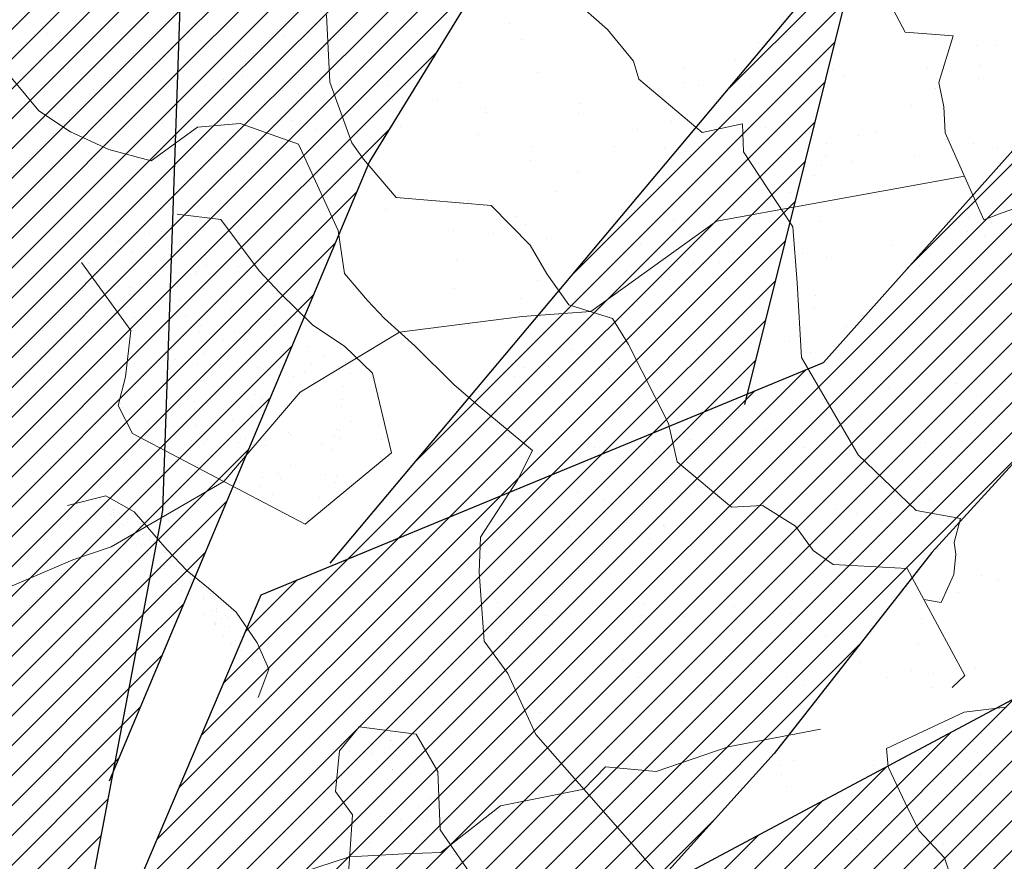
# Model space of a CAD drawing. Units: inches. Extents: x 1986 to 21484, y -1816 to 2016.
# Tile 73 of 85: x 3669.485 to 3676.656, y 1888.787 to 1894.917. Entities that reach past the tile are written whole.
import ezdxf

# ---------------------------------------------------------------- set-up
doc = ezdxf.new("R2010")
doc.units = ezdxf.units.IN
doc.layers.add('L-PLNT', color=84, linetype='Continuous', lineweight=13)
doc.layers.add('vfolhas', color=114, linetype='Continuous', lineweight=5)
doc.layers.add('vfolha2', color=110, linetype='Continuous')
doc.layers.add('vfolhas2', color=102, linetype='Continuous')
pattern_1 = [(45, (-2446.5133113, 50.986076), (-0.004419417382, 0.004419417382), [])]

# ---------------------------------------------------------------- blocks, each defined once
blk = doc.blocks.new('arbusto_PB_verde_grande')
at = {"layer": 'vfolha2'}
h = blk.add_hatch(dxfattribs=at)
h.set_pattern_fill('ANSI31', color=256, scale=0.05, style=0)
h.set_pattern_definition(pattern_1)
h.paths.add_polyline_path([(0.02944, 0.35651), (0.00028, 0.09048), (0.02625, -0.03934), (0.047, 0.06233), (0.06189, 0.09731), (0.09372, 0.26573), (0.09955, 0.43473), (0.08789, 0.61313), (0.0645, 0.72266), (0.04988, 0.6851), (0.0236, 0.51294)])
h.paths.add_polyline_path([(0.30106, 0.43789), (0.14225, 0.24871), (0.26685, 0.30022)])
h.paths.add_polyline_path([(0.37995, 0.22817), (0.23697, 0.15193), (0.18428, 0.09364), (0.11122, 0.04358), (0.02625, -0.03934), (0.28061, 0.04667), (0.36829, 0.07798), (0.46756, 0.11239), (0.61068, 0.19376), (0.71585, 0.27823), (0.55813, 0.25948)])
h.paths.add_polyline_path([(0.56101, -0.29441), (0.72752, -0.32573), (0.59024, -0.2412), (0.42962, -0.15982), (0.02625, -0.03934), (0.14922, -0.14107), (0.18838, -0.16604), (0.41501, -0.24435)])
h.paths.add_polyline_path([(-0.27429, -0.44776), (-0.30352, -0.72628), (-0.23923, -0.64175), (-0.15457, -0.45716), (0.02625, -0.03934), (-0.16328, -0.25376)])
h.paths.add_polyline_path([(-0.51963, -0.24744), (-0.67736, -0.32573), (-0.59558, -0.35072), (-0.40574, -0.32882), (-0.21007, -0.20995), (0.02625, -0.03934), (-0.14874, -0.06595), (-0.31518, -0.09101), (-0.41452, -0.15048)])
h.paths.add_polyline_path([(-0.52546, 0.25007), (-0.70947, 0.24698), (-0.51963, 0.1093), (-0.32979, 0.02167), (-0.07567, -0.0128), (-0.04234, -0.02148), (-0.35024, 0.1312)])
at = {"layer": 'vfolhas'}
h = blk.add_hatch(dxfattribs=at)
h.set_pattern_fill('ANSI31', color=256, scale=0.05, style=0)
h.set_pattern_definition(pattern_1)
h.paths.add_polyline_path([(-0.07279, 0.50669), (-0.18085, 0.65063), (-0.2334, 0.67253), (-0.20712, 0.53176), (-0.10785, 0.25007), (0.02625, -0.03934), (0.00028, 0.09048), (0.00816, 0.16241), (-0.04939, 0.29079)])
h.paths.add_polyline_path([(0.09902, 0.41929), (0.09372, 0.26573), (0.07906, 0.18814), (0.15506, 0.36901), (0.26606, 0.5505), (0.28356, 0.63504), (0.2485, 0.68819), (0.25145, 0.63504), (0.20178, 0.54426)])
h.paths.add_polyline_path([(0.12295, 0.24073), (0.047, 0.06233), (0.02625, -0.03934), (0.11122, 0.04358), (0.18428, 0.09364), (0.27478, 0.19376), (0.3215, 0.25323), (0.44129, 0.38467), (0.47634, 0.57866), (0.41789, 0.45347), (0.28939, 0.30954)])
h.paths.add_polyline_path([(0.58145, -0.03779), (0.70707, 0.01536), (0.78591, 0.04667), (0.74796, 0.06549), (0.62818, 0.08423), (0.52595, 0.09048), (0.39745, 0.04358), (0.02625, -0.03934), (0.25728, -0.03154), (0.43834, -0.0347)])
h.paths.add_polyline_path([(0.52022, -0.03647), (0.43834, -0.0347), (0.25728, -0.03154), (0.02625, -0.03934), (0.17964, -0.08515), (0.53768, -0.13167), (0.69541, -0.15357), (0.78591, -0.07852), (0.70413, -0.10042)])
h.paths.add_polyline_path([(0.27189, -0.21929), (0.14922, -0.14107), (0.02625, -0.03934), (0.15794, -0.31007), (0.29522, -0.42585), (0.41789, -0.49157), (0.56396, -0.56669), (0.5114, -0.48532), (0.39456, -0.34139)])
h.paths.add_polyline_path([(-0.05818, -0.47591), (-0.02312, -0.61984), (0.047, -0.80134), (0.08494, -0.59794), (0.07911, -0.4071), (0.03527, -0.25376), (0.02625, -0.03934), (-0.03773, -0.26001)])
h.paths.add_polyline_path([(-0.24218, 0.14054), (-0.11073, 0.06858), (0.02625, -0.03934), (-0.04235, 0.10871), (-0.21007, 0.23757), (-0.36485, 0.33145), (-0.47874, 0.40341), (-0.54303, 0.46288), (-0.49041, 0.33145), (-0.39408, 0.22192)])
at = {"layer": 'vfolha2'}
for p, q in [((0.14339, 0.25007), (0.30106, 0.43789)), ((0.30106, 0.43789), (0.26606, 0.29704)), ((0.09955, 0.43473), (0.09372, 0.26573)), ((0.23697, 0.15193), (0.37995, 0.22817))]:
    blk.add_line(p, q, dxfattribs=at)
at = {"layer": 'vfolhas2'}
for p, q in [((0.26606, 0.5505), (0.15506, 0.36901)), ((0.28939, 0.30954), (0.41789, 0.45347)), ((0.44129, 0.38467), (0.3215, 0.25323)), ((0.15506, 0.36901), (0.07795, 0.18551)), ((0.12295, 0.24073), (0.28939, 0.30954)), ((0.09372, 0.26573), (0.06189, 0.09731)), ((0.3215, 0.25323), (0.27478, 0.19376)), ((0.047, 0.06233), (0.12295, 0.24073)), ((0.27478, 0.19376), (0.18428, 0.09364))]:
    blk.add_line(p, q, dxfattribs=at)
blk = doc.blocks.new('PLANT-SHRUB')
for p, q in [((2155.3771, 1891.3729), (2155.4666, 1891.568)), ((2155.3771, 1891.1047), (2155.3771, 1891.3729)), ((2155.3155, 1891.2998), (2155.3155, 1891.2998)), ((2154.9383, 1891.2139), (2154.9383, 1891.2139)), ((2155.4084, 1891.1607), (2155.4084, 1891.1607)), ((2154.7698, 1891.1065), (2154.7698, 1891.1065)), ((2155.3283, 1890.934), (2155.3771, 1891.1047)), ((2155.3348, 1891.0932), (2155.3348, 1891.0932)), ((2154.6758, 1890.9774), (2154.6758, 1890.9774)), ((2155.2225, 1890.6089), (2155.3283, 1890.934)), ((2154.3034, 1890.8771), (2154.5474, 1890.6983)), ((2154.8084, 1890.8995), (2154.8084, 1890.8995)), ((2155.2187, 1890.9059), (2155.2187, 1890.9059)), ((2155.4267, 1890.8785), (2155.4267, 1890.8785)), ((2155.8546, 1890.8861), (2155.8546, 1890.8861)), ((2155.7517, 1890.8357), (2155.7517, 1890.8357)), ((2154.937, 1890.7286), (2154.937, 1890.7286)), ((2154.5474, 1890.6983), (2155.1412, 1890.5032)), ((2155.1412, 1890.5032), (2155.2225, 1890.6089)), ((2155.2223, 1890.5996), (2155.2223, 1890.5996)), ((2154.1988, 1889.8984), (2154.3599, 1890.5058)), ((2154.268, 1890.5248), (2154.268, 1890.5248)), ((2154.3599, 1890.5058), (2154.4874, 1890.5058)), ((2154.3599, 1890.5058), (2154.3599, 1890.5058)), ((2155.2904, 1890.5297), (2155.2904, 1890.5297)), ((2154.5893, 1890.41), (2154.5893, 1890.41)), ((2156.1384, 1890.3779), (2156.1384, 1890.3779)), ((2154.5156, 1890.3425), (2154.5156, 1890.3425)), ((2154.6155, 1890.2131), (2154.6155, 1890.2131)), ((2155.8602, 1890.2108), (2155.8602, 1890.2108)), ((2153.7037, 1890.1683), (2153.7037, 1890.1683)), ((2154.447, 1890.1057), (2154.447, 1890.1057)), ((2154.7832, 1890.1294), (2154.7832, 1890.1294)), ((2155.9718, 1889.7054), (2155.3949, 1890.0722)), ((2155.6916, 1890.1034), (2155.6916, 1890.1034)), ((2155.8294, 1890.1161), (2155.8294, 1890.1161)), ((2153.7744, 1890.0612), (2153.7744, 1890.0612)), ((2153.9153, 1889.9136), (2154.1228, 1889.9996)), ((2153.9824, 1890.0338), (2153.9824, 1890.0338)), ((2154.1228, 1889.9996), (2154.1988, 1889.8984)), ((2155.7907, 1890.0592), (2155.7907, 1890.0592)), ((2156.968, 1889.7436), (2156.9795, 1890.0186)), ((2154.1178, 1889.978), (2154.1178, 1889.978)), ((2154.3073, 1889.9911), (2154.3073, 1889.9911)), ((2155.7171, 1889.9917), (2155.7171, 1889.9917)), ((2153.8039, 1889.8174), (2153.9153, 1889.9136)), ((2154.1988, 1889.8984), (2154.1324, 1889.6508)), ((2154.8502, 1889.9196), (2154.8502, 1889.9196)), ((2155.0582, 1889.8922), (2155.0582, 1889.8922)), ((2155.3832, 1889.8494), (2155.3832, 1889.8494)), ((2153.7533, 1889.7466), (2153.8039, 1889.8174)), ((2155.926, 1889.778), (2155.926, 1889.778)), ((2153.6014, 1889.6505), (2153.7533, 1889.7466)), ((2154.2428, 1889.7547), (2154.2428, 1889.7547)), ((2155.2652, 1889.7596), (2155.2652, 1889.7596)), ((2156.1341, 1889.7506), (2156.1341, 1889.7506)), ((2156.3446, 1889.7207), (2156.3446, 1889.7207)), ((2156.459, 1889.7078), (2156.459, 1889.7078)), ((2156.9323, 1888.68), (2156.968, 1889.7436)), ((2153.7961, 1889.386), (2153.6014, 1889.6505)), ((2153.7701, 1889.6594), (2153.7701, 1889.6594)), ((2154.1324, 1889.6508), (2154.5056, 1889.2597)), ((2156.4787, 1889.4784), (2155.9718, 1889.7054)), ((2153.6549, 1889.6011), (2153.6549, 1889.6011)), ((2153.6964, 1889.5919), (2153.6964, 1889.5919)), ((2154.8995, 1889.5988), (2154.8995, 1889.5988)), ((2155.3193, 1889.6272), (2155.3193, 1889.6272)), ((2156.1441, 1889.5965), (2156.1441, 1889.5965)), ((2156.7234, 1889.1989), (2156.4787, 1889.4784)), ((2153.6786, 1889.3982), (2153.6786, 1889.3982)), ((2153.8268, 1888.8023), (2153.7961, 1889.386)), ((2154.758, 1889.3593), (2154.758, 1889.3593)), ((2154.9715, 1889.3086), (2154.9715, 1889.3086)), ((2155.8042, 1889.346), (2155.8042, 1889.346)), ((2156.5207, 1889.2764), (2156.5207, 1889.2764)), ((2153.0481, 1889.2145), (2153.0481, 1889.2145)), ((2153.2986, 1889.2274), (2153.2986, 1889.2274)), ((2154.2928, 1889.2123), (2154.2928, 1889.2123)), ((2154.5056, 1889.2597), (2154.542, 1889.0869)), ((2154.8979, 1889.2411), (2154.8979, 1889.2411)), ((2155.5374, 1889.21), (2155.5374, 1889.21)), ((2156.9502, 1889.2118), (2156.7234, 1889.1989)), ((2156.782, 1889.2077), (2156.782, 1889.2077)), ((2157.475, 1888.8845), (2156.9502, 1889.2118)), ((2152.863, 1889.1464), (2152.863, 1889.1464)), ((2157.9168, 1888.7107), (2157.9866, 1889.1716)), ((2152.8796, 1889.1072), (2152.8796, 1889.1072)), ((2153.4059, 1889.0749), (2153.4059, 1889.0749)), ((2154.1242, 1889.1049), (2154.1242, 1889.1049)), ((2154.542, 1889.0869), (2154.5147, 1888.8686)), ((2155.3689, 1889.1026), (2155.3689, 1889.1026)), ((2156.6135, 1889.1004), (2156.6135, 1889.1004)), ((2153.1714, 1888.9979), (2153.1714, 1888.9979)), ((2153.6139, 1889.0475), (2153.6139, 1889.0475)), ((2153.9388, 1889.0048), (2153.9388, 1889.0048)), ((2155.24, 1888.9895), (2155.24, 1888.9895)), ((2154.2176, 1888.9846), (2154.2176, 1888.9846)), ((2154.4817, 1888.9333), (2154.4817, 1888.9333)), ((2156.173, 1888.9578), (2156.173, 1888.9578)), ((2156.3195, 1888.9506), (2156.3195, 1888.9506)), ((2157.993, 1888.9486), (2157.993, 1888.9486)), ((2152.9509, 1888.9087), (2152.9509, 1888.9087)), ((2154.5001, 1888.8766), (2154.5001, 1888.8766)), ((2154.5147, 1888.8686), (2154.5875, 1888.5957)), ((2154.6897, 1888.9059), (2154.6897, 1888.9059)), ((2155.0147, 1888.8631), (2155.0147, 1888.8631)), ((2156.0993, 1888.8903), (2156.0993, 1888.8903)), ((2158.0239, 1888.8339), (2157.475, 1888.8845)), ((2157.9562, 1888.9149), (2157.9562, 1888.9149)), ((2152.8772, 1888.8412), (2152.8772, 1888.8412)), ((2153.6423, 1888.0035), (2153.8268, 1888.8023)), ((2155.5575, 1888.7917), (2155.5575, 1888.7917)), ((2158.2267, 1888.6574), (2158.0239, 1888.8339)), ((2155.7656, 1888.7643), (2155.7656, 1888.7643)), ((2156.0905, 1888.7215), (2156.0905, 1888.7215)), ((2157.6372, 1888.3894), (2157.9168, 1888.7107)), ((2158.1345, 1888.742), (2158.1345, 1888.742)), ((2156.6334, 1888.65), (2156.6334, 1888.65)), ((2156.7781, 1888.2176), (2156.9323, 1888.68)), ((2158.0268, 1888.6514), (2158.0268, 1888.6514)), ((2158.5318, 1888.4034), (2158.2267, 1888.6574)), ((2152.631, 1888.6232), (2152.631, 1888.6232)), ((2153.3321, 1888.6002), (2153.3321, 1888.6002)), ((2153.6534, 1888.6281), (2153.6534, 1888.6281)), ((2154.5767, 1888.598), (2154.5767, 1888.598)), ((2154.5875, 1888.5957), (2154.7604, 1888.4502)), ((2154.7329, 1888.5892), (2154.7329, 1888.5892)), ((2155.779, 1888.5759), (2155.779, 1888.5759)), ((2155.8214, 1888.5957), (2155.8214, 1888.5957)), ((2156.8014, 1888.5808), (2156.8014, 1888.5808)), ((2156.8414, 1888.6226), (2156.8414, 1888.6226)), ((2157.9425, 1888.5977), (2157.9425, 1888.5977)), ((2158.7555, 1888.6129), (2158.3082, 1888.1939)), ((2154.0787, 1888.4905), (2154.0787, 1888.4905)), ((2154.1524, 1888.558), (2154.1524, 1888.558)), ((2155.7015, 1888.5258), (2155.7015, 1888.5258)), ((2157.8132, 1888.4947), (2157.8132, 1888.4947)), ((2157.8809, 1888.5419), (2157.8809, 1888.5419)), ((2158.358, 1888.5572), (2158.358, 1888.5572)), ((2158.404, 1888.5352), (2158.404, 1888.5352)), ((2152.4794, 1888.4767), (2152.4794, 1888.4767)), ((2154.7604, 1888.4502), (2154.8241, 1887.9369)), ((2154.7604, 1888.4502), (2154.7604, 1888.4502)), ((2157.9172, 1888.481), (2157.9172, 1888.481)), ((2158.0797, 1888.4596), (2158.0797, 1888.4596)), ((2158.3511, 1888.4239), (2158.3511, 1888.4239)), ((2151.8639, 1888.2323), (2151.4605, 1888.408)), ((2157.5673, 1888.0821), (2157.6372, 1888.3894)), ((2158.1219, 1888.357), (2158.1219, 1888.357)), ((2158.1473, 1888.3641), (2158.1473, 1888.3641)), ((2158.1688, 1888.3442), (2158.1688, 1888.3442)), ((2158.1842, 1888.3979), (2158.1842, 1888.3979)), ((2158.4551, 1888.4102), (2158.4551, 1888.4102)), ((2159.4328, 1887.9763), (2158.5318, 1888.4034)), ((2151.9879, 1888.1806), (2151.8639, 1888.2323)), ((2151.9616, 1888.2303), (2151.9616, 1888.2303)), ((2152.0668, 1888.2667), (2152.0668, 1888.2667)), ((2152.1696, 1888.2029), (2152.1696, 1888.2029)), ((2152.7253, 1888.2137), (2152.7253, 1888.2137)), ((2153.1463, 1888.2278), (2153.1463, 1888.2278)), ((2153.97, 1888.2114), (2153.97, 1888.2114)), ((2154.1924, 1888.2145), (2154.1924, 1888.2145)), ((2155.2146, 1888.2092), (2155.2146, 1888.2092)), ((2155.2148, 1888.2194), (2155.2148, 1888.2194)), ((2155.3538, 1888.2072), (2155.3538, 1888.2072)), ((2156.4592, 1888.2069), (2156.4592, 1888.2069)), ((2156.7418, 1887.9274), (2156.7781, 1888.2176)), ((2156.7781, 1888.2176), (2156.7781, 1888.2176)), ((2151.7601, 1887.5256), (2151.9879, 1888.1806)), ((2152.1317, 1888.1581), (2152.1317, 1888.1581)), ((2152.4945, 1888.1601), (2152.4945, 1888.1601)), ((2155.2802, 1888.1397), (2155.2802, 1888.1397)), ((2156.2943, 1888.1805), (2156.2943, 1888.1805)), ((2157.8654, 1888.151), (2157.8654, 1888.151)), ((2157.8683, 1888.1568), (2157.8683, 1888.1568)), ((2157.9484, 1888.1819), (2157.9484, 1888.1819)), ((2158.3082, 1888.1939), (2158.2802, 1887.9844)), ((2152.0581, 1888.0906), (2152.0581, 1888.0906)), ((2152.5568, 1888.1063), (2152.5568, 1888.1063)), ((2153.0374, 1888.0886), (2153.0374, 1888.0886)), ((2153.2454, 1888.0613), (2153.2454, 1888.0613)), ((2153.6809, 1888.1259), (2153.6809, 1888.1259)), ((2153.8014, 1888.1041), (2153.8014, 1888.1041)), ((2155.0461, 1888.1018), (2155.0461, 1888.1018)), ((2156.2907, 1888.0996), (2156.2907, 1888.0996)), ((2157.8329, 1887.7609), (2157.5673, 1888.0821)), ((2157.7811, 1888.0973), (2157.7811, 1888.0973)), ((2153.2939, 1887.5837), (2153.6423, 1888.0035)), ((2153.5703, 1888.0185), (2153.5703, 1888.0185)), ((2157.733, 1887.9879), (2157.733, 1887.9879)), ((2157.7377, 1887.9888), (2157.7377, 1887.9888)), ((2157.7746, 1888.0226), (2157.7746, 1888.0226)), ((2154.1132, 1887.947), (2154.1132, 1887.947)), ((2154.3212, 1887.9196), (2154.3212, 1887.9196)), ((2154.8241, 1887.9369), (2154.6784, 1887.6913)), ((2156.4241, 1887.5374), (2156.7418, 1887.9274)), ((2157.8954, 1887.9665), (2157.8954, 1887.9665)), ((2158.2802, 1887.9844), (2158.0565, 1887.7888)), ((2158.1093, 1887.9719), (2158.1093, 1887.9719)), ((2158.1669, 1887.9307), (2158.1669, 1887.9307)), ((2151.5596, 1887.8664), (2151.5596, 1887.8664)), ((2151.874, 1887.8531), (2153.4137, 1886.8553)), ((2152.6058, 1887.8531), (2152.6058, 1887.8531)), ((2153.6282, 1887.858), (2153.6282, 1887.858)), ((2154.6462, 1887.8768), (2154.6462, 1887.8768)), ((2156.5553, 1887.8564), (2156.5553, 1887.8564)), ((2158.0074, 1887.8438), (2158.0074, 1887.8438)), ((2153.3332, 1887.8073), (2153.3332, 1887.8073)), ((2154.7077, 1887.8191), (2154.7077, 1887.8191)), ((2154.8824, 1887.7752), (2154.8824, 1887.7752)), ((2155.189, 1887.8054), (2155.189, 1887.8054)), ((2155.3971, 1887.778), (2155.3971, 1887.778)), ((2155.7539, 1887.8058), (2155.7539, 1887.8058)), ((2156.4816, 1887.7889), (2156.4816, 1887.7889)), ((2158.0565, 1887.7888), (2157.8329, 1887.7609)), ((2157.8557, 1887.7718), (2157.8557, 1887.7718)), ((2151.6603, 1887.7261), (2151.6603, 1887.7261)), ((2153.2595, 1887.7398), (2153.2595, 1887.7398)), ((2155.722, 1887.7352), (2155.722, 1887.7352)), ((2154.6784, 1887.6913), (2154.4964, 1887.0728)), ((2156.2649, 1887.6637), (2156.2649, 1887.6637)), ((2151.7647, 1887.6017), (2151.7647, 1887.6017)), ((2153.0093, 1887.5994), (2153.0093, 1887.5994)), ((2153.0377, 1887.2662), (2153.2939, 1887.5837)), ((2153.2939, 1887.5837), (2153.2939, 1887.5837)), ((2154.2539, 1887.5972), (2154.2539, 1887.5972)), ((2155.4986, 1887.5949), (2155.4986, 1887.5949)), ((2151.636, 1887.381), (2151.7601, 1887.5256)), ((2151.7601, 1887.5256), (2151.7601, 1887.5256)), ((2152.0416, 1887.4966), (2152.0416, 1887.4966)), ((2156.2426, 1887.3561), (2156.4241, 1887.5374)), ((2153.1211, 1887.4577), (2153.1211, 1887.4577)), ((2154.1673, 1887.4444), (2154.1673, 1887.4444)), ((2154.5346, 1887.4565), (2154.5346, 1887.4565)), ((2155.1896, 1887.4493), (2155.1896, 1887.4493)), ((2151.2389, 1887.34), (2151.2389, 1887.34)), ((2151.3125, 1887.4075), (2151.3125, 1887.4075)), ((2151.543, 1887.226), (2151.636, 1887.381)), ((2152.8617, 1887.3753), (2152.8617, 1887.3753)), ((2154.461, 1887.389), (2154.461, 1887.389)), ((2155.7616, 1887.2382), (2156.2426, 1887.3561)), ((2156.2426, 1887.3561), (2156.2426, 1887.3561)), ((2151.0502, 1887.3155), (2151.0502, 1887.3155)), ((2151.1579, 1887.2152), (2151.1579, 1887.2152)), ((2151.2327, 1887.0503), (2151.543, 1887.226)), ((2151.5931, 1887.244), (2151.5931, 1887.244)), ((2151.8011, 1887.2166), (2151.8011, 1887.2166)), ((2152.4026, 1887.2129), (2152.4026, 1887.2129)), ((2152.9249, 1886.6211), (2153.0377, 1887.2662)), ((2153.6472, 1887.2106), (2153.6472, 1887.2106)), ((2154.8918, 1887.2084), (2154.8918, 1887.2084)), ((2155.5347, 1887.1566), (2155.7616, 1887.2382)), ((2152.126, 1887.1738), (2152.126, 1887.1738)), ((2155.5986, 1886.6458), (2155.5347, 1887.1566)), ((2151.5345, 1887.0963), (2151.5345, 1887.0963)), ((2152.234, 1887.1055), (2152.234, 1887.1055)), ((2152.514, 1887.0567), (2152.514, 1887.0567)), ((2152.5806, 1887.083), (2152.5806, 1887.083)), ((2152.6689, 1887.1023), (2152.6689, 1887.1023)), ((2152.8769, 1887.075), (2152.8769, 1887.075)), ((2153.4787, 1887.1033), (2153.4787, 1887.1033)), ((2153.603, 1887.0879), (2153.603, 1887.0879)), ((2154.4964, 1887.0728), (2154.4509, 1886.8545)), ((2154.7233, 1887.101), (2154.7233, 1887.101)), ((2158.0257, 1887.0028), (2158.2229, 1887.1013)), ((2151.4706, 1886.7919), (2151.2327, 1887.0503)), ((2152.4403, 1886.9892), (2152.4403, 1886.9892)), ((2153.2019, 1887.0322), (2153.2019, 1887.0322)), ((2154.0632, 1887.0245), (2154.0632, 1887.0245)), ((2154.6825, 1887.049), (2154.6825, 1887.049)), ((2157.9553, 1886.8057), (2158.0257, 1887.0028)), ((2158.0257, 1887.0028), (2158.0257, 1887.0028)), ((2153.7447, 1886.9607), (2153.7447, 1886.9607)), ((2153.9528, 1886.9333), (2153.9528, 1886.9333)), ((2153.4137, 1886.8553), (2154.5328, 1886.7089)), ((2154.2777, 1886.8905), (2154.2777, 1886.8905)), ((2154.4509, 1886.8545), (2154.6147, 1886.5634)), ((2158.0715, 1886.8795), (2158.0715, 1886.8795)), ((2151.2728, 1886.0864), (2151.4706, 1886.7919)), ((2154.8205, 1886.8191), (2154.8205, 1886.8191)), ((2155.0286, 1886.7917), (2155.0286, 1886.7917)), ((2157.913, 1886.5383), (2157.9553, 1886.8057)), ((2158.082, 1886.7676), (2158.082, 1886.7676)), ((2158.0892, 1886.8298), (2158.0892, 1886.8298)), ((2152.0164, 1886.7265), (2152.0164, 1886.7265)), ((2153.7155, 1886.7059), (2153.7155, 1886.7059)), ((2154.5328, 1886.7089), (2154.9211, 1886.3936)), ((2155.3535, 1886.7489), (2155.3535, 1886.7489)), ((2158.003, 1886.6952), (2158.003, 1886.6952)), ((2158.0168, 1886.7078), (2158.0168, 1886.7078)), ((2158.0245, 1886.7223), (2158.0245, 1886.7223)), ((2158.0426, 1886.712), (2158.0426, 1886.712)), ((2152.0425, 1886.6247), (2152.0425, 1886.6247)), ((2153.0959, 1886.6876), (2153.0959, 1886.6876)), ((2153.6418, 1886.6384), (2153.6418, 1886.6384)), ((2154.1421, 1886.6743), (2154.1421, 1886.6743)), ((2155.1645, 1886.6792), (2155.1645, 1886.6792)), ((2155.2646, 1886.6737), (2155.2646, 1886.6737)), ((2155.6244, 1886.4136), (2155.5986, 1886.6458)), ((2158.011, 1886.6919), (2158.011, 1886.6919)), ((2158.0553, 1886.6852), (2158.0553, 1886.6852)), ((2158.0943, 1886.6801), (2158.0943, 1886.6801)), ((2152.6865, 1886.5986), (2152.6865, 1886.5986)), ((2152.7917, 1886.4675), (2152.9249, 1886.6211)), ((2153.9312, 1886.5963), (2153.9312, 1886.5963)), ((2154.6147, 1886.5634), (2154.5783, 1886.2905)), ((2155.1758, 1886.5941), (2155.1758, 1886.5941)), ((2158.0198, 1886.5779), (2158.0198, 1886.5779)), ((2158.0958, 1886.5969), (2158.0958, 1886.5969)), ((2157.9412, 1886.2708), (2157.913, 1886.5383)), ((2157.9821, 1886.5244), (2157.9821, 1886.5244)), ((2157.9862, 1886.5003), (2157.9862, 1886.5003)), ((2158.0252, 1886.4952), (2158.0252, 1886.4952)), ((2158.0747, 1886.4887), (2158.0747, 1886.4887)), ((2158.0861, 1886.4872), (2158.0861, 1886.4872)), ((2158.0885, 1886.5014), (2158.0885, 1886.5014)), ((2152.7917, 1886.4675), (2152.7917, 1886.4675)), ((2153.0479, 1886.3139), (2152.7917, 1886.4675)), ((2155.6373, 1886.0136), (2155.6244, 1886.4136)), ((2156.2958, 1886.4652), (2155.9988, 1885.9491)), ((2156.4895, 1886.4523), (2156.2958, 1886.4652)), ((2157.1093, 1886.4136), (2156.4895, 1886.4523)), ((2157.3288, 1885.7813), (2157.1093, 1886.4136)), ((2158.0001, 1886.4204), (2158.0001, 1886.4204)), ((2158.0151, 1886.4336), (2158.0151, 1886.4336)), ((2158.0353, 1886.4092), (2158.0353, 1886.4092)), ((2154.9169, 1886.3551), (2154.9169, 1886.3551)), ((2154.9211, 1886.3936), (2155.6502, 1885.8652)), ((2156.2786, 1886.3449), (2156.2786, 1886.3449)), ((2156.7369, 1886.3459), (2156.7369, 1886.3459)), ((2156.9009, 1886.3437), (2156.9009, 1886.3437)), ((2158.0948, 1886.389), (2158.0948, 1886.389)), ((2152.5555, 1886.3129), (2152.5555, 1886.3129)), ((2153.1193, 1885.7143), (2153.0479, 1886.3139)), ((2153.244, 1886.2739), (2153.244, 1886.2739)), ((2153.5779, 1886.3178), (2153.5779, 1886.3178)), ((2154.5783, 1886.2905), (2154.5237, 1886.054)), ((2154.6573, 1886.2789), (2154.6573, 1886.2789)), ((2154.8433, 1886.2876), (2154.8433, 1886.2876)), ((2156.7001, 1886.3122), (2156.7001, 1886.3122)), ((2157.9412, 1886.2708), (2157.9412, 1886.2708)), ((2157.9694, 1886.0738), (2157.9412, 1886.2708)), ((2157.9561, 1886.3103), (2157.9561, 1886.3103)), ((2158.0104, 1886.2892), (2158.0104, 1886.2892)), ((2158.017, 1886.3023), (2158.017, 1886.3023)), ((2152.0798, 1886.2121), (2152.0798, 1886.2121)), ((2153.3244, 1886.2098), (2153.3244, 1886.2098)), ((2154.569, 1886.2075), (2154.569, 1886.2075)), ((2156.2313, 1886.2553), (2156.2313, 1886.2553)), ((2156.7544, 1886.2486), (2156.7544, 1886.2486)), ((2157.9659, 1886.2435), (2157.9659, 1886.2435)), ((2157.9748, 1886.2216), (2157.9748, 1886.2216)), ((2158.0718, 1886.2139), (2158.0718, 1886.2139)), ((2156.5012, 1886.1299), (2156.5012, 1886.1299)), ((2156.5975, 1886.1505), (2156.5975, 1886.1505)), ((2157.9928, 1886.1415), (2157.9928, 1886.1415)), ((2158.0056, 1886.1448), (2158.0056, 1886.1448)), ((2158.0066, 1886.1542), (2158.0066, 1886.1542)), ((2158.0628, 1886.1286), (2158.0628, 1886.1286)), ((2158.0944, 1886.1487), (2158.0944, 1886.1487)), ((2152.3004, 1886.1161), (2152.3004, 1886.1161)), ((2152.5084, 1886.0887), (2152.5084, 1886.0887)), ((2153.1559, 1886.1024), (2153.1559, 1886.1024)), ((2154.4005, 1886.1002), (2154.4005, 1886.1002)), ((2154.5237, 1886.054), (2154.5332, 1885.65)), ((2156.354, 1886.0998), (2156.354, 1886.0998)), ((2156.4581, 1886.0861), (2156.4581, 1886.0861)), ((2156.4723, 1886.0703), (2156.4723, 1886.0703)), ((2156.5132, 1886.0968), (2156.5132, 1886.0968)), ((2156.6205, 1886.0647), (2156.6205, 1886.0647)), ((2157.0121, 1886.0509), (2157.0121, 1886.0509)), ((2157.1356, 1886.0957), (2157.1356, 1886.0957)), ((2157.9694, 1885.8626), (2157.9694, 1886.0738)), ((2158.0497, 1886.104), (2158.0497, 1886.104)), ((2158.0887, 1886.0989), (2158.0887, 1886.0989)), ((2152.8334, 1886.0459), (2152.8334, 1886.0459)), ((2155.6631, 1885.7168), (2155.6373, 1886.0136)), ((2156.892, 1886.029), (2156.892, 1886.029)), ((2156.996, 1886.0153), (2156.996, 1886.0153)), ((2157.1584, 1885.9939), (2157.1584, 1885.9939)), ((2158.0009, 1886.0005), (2158.0009, 1886.0005)), ((2152.8963, 1885.9553), (2152.8963, 1885.9553)), ((2153.0707, 1885.9175), (2153.0707, 1885.9175)), ((2153.3762, 1885.9744), (2153.3762, 1885.9744)), ((2153.5843, 1885.947), (2153.5843, 1885.947)), ((2154.4455, 1885.9231), (2154.4455, 1885.9231)), ((2155.1393, 1885.9091), (2155.1393, 1885.9091)), ((2155.9988, 1885.9491), (2156.0118, 1885.6652)), ((2156.2905, 1885.9368), (2156.2905, 1885.9368)), ((2156.3274, 1885.9706), (2156.3274, 1885.9706)), ((2157.1019, 1885.9545), (2157.1019, 1885.9545)), ((2157.9806, 1885.9191), (2157.9806, 1885.9191)), ((2158.0023, 1885.941), (2158.0023, 1885.941)), ((2158.0196, 1885.914), (2158.0196, 1885.914)), ((2158.0196, 1885.914), (2158.0196, 1885.914)), ((2158.0339, 1885.9611), (2158.0339, 1885.9611)), ((2158.0645, 1885.9351), (2158.0645, 1885.9351)), ((2158.0783, 1885.9477), (2158.0783, 1885.9477)), ((2158.0805, 1885.9059), (2158.0805, 1885.9059)), ((2158.0975, 1885.9263), (2158.0975, 1885.9263)), ((2152.8226, 1885.8878), (2152.8226, 1885.8878)), ((2153.9092, 1885.9043), (2153.9092, 1885.9043)), ((2154.1169, 1885.9042), (2154.1169, 1885.9042)), ((2155.6502, 1885.8652), (2156.4772, 1885.6891)), ((2156.1172, 1885.8445), (2156.1172, 1885.8445)), ((2156.2188, 1885.8702), (2156.2188, 1885.8702)), ((2156.7395, 1885.8433), (2156.7395, 1885.8433)), ((2156.7418, 1885.8635), (2156.7418, 1885.8635)), ((2157.253, 1885.866), (2157.253, 1885.866)), ((2157.9553, 1885.4967), (2157.9694, 1885.8626)), ((2157.9899, 1885.8667), (2157.9899, 1885.8667)), ((2157.9962, 1885.8561), (2157.9962, 1885.8561)), ((2158.0871, 1885.846), (2158.0871, 1885.846)), ((2154.452, 1885.8328), (2154.452, 1885.8328)), ((2154.6601, 1885.8054), (2154.6601, 1885.8054)), ((2154.985, 1885.7626), (2154.985, 1885.7626)), ((2156.4772, 1885.6891), (2157.3288, 1885.7813)), ((2156.9281, 1885.7952), (2156.9281, 1885.7952)), ((2157.3288, 1885.7813), (2158.2522, 1885.5676)), ((2157.5742, 1885.0717), (2157.3288, 1885.7813)), ((2157.9734, 1885.7735), (2157.9734, 1885.7735)), ((2158.0928, 1885.782), (2158.0928, 1885.782)), ((2158.0928, 1885.782), (2158.0928, 1885.782)), ((2153.0578, 1885.5914), (2153.1193, 1885.7143)), ((2153.1193, 1885.7143), (2153.1193, 1885.7143)), ((2155.6631, 1885.5362), (2155.6631, 1885.7168)), ((2156.0916, 1885.7546), (2156.0916, 1885.7546)), ((2156.8913, 1885.7615), (2156.8913, 1885.7615)), ((2157.9915, 1885.7117), (2157.9915, 1885.7117)), ((2158.0115, 1885.7211), (2158.0115, 1885.7211)), ((2158.0856, 1885.7095), (2158.0856, 1885.7095)), ((2154.5332, 1885.65), (2154.9975, 1885.1315)), ((2156.0118, 1885.6652), (2156.0763, 1885.3943)), ((2156.4361, 1885.6501), (2156.4361, 1885.6501)), ((2156.4597, 1885.6853), (2156.4597, 1885.6853)), ((2156.9995, 1885.6658), (2156.9995, 1885.6658)), ((2157.0584, 1885.6489), (2157.0584, 1885.6489)), ((2158.0066, 1885.6591), (2158.0066, 1885.6591)), ((2158.0266, 1885.6584), (2158.0266, 1885.6584)), ((2158.0616, 1885.6602), (2158.0616, 1885.6602)), ((2158.0881, 1885.6376), (2158.0881, 1885.6376)), ((2153.0373, 1885.2944), (2153.0578, 1885.5914)), ((2153.5527, 1885.5477), (2153.5527, 1885.5477)), ((2153.6084, 1885.5955), (2153.6084, 1885.5955)), ((2154.0978, 1885.6045), (2154.0978, 1885.6045)), ((2154.853, 1885.5933), (2154.853, 1885.5933)), ((2156.1698, 1885.6066), (2156.1698, 1885.6066)), ((2156.2738, 1885.5929), (2156.2738, 1885.5929)), ((2156.3519, 1885.5964), (2156.3519, 1885.5964)), ((2156.4363, 1885.5716), (2156.4363, 1885.5716)), ((2156.6924, 1885.5792), (2156.6924, 1885.5792)), ((2156.9742, 1885.5952), (2156.9742, 1885.5952)), ((2157.9826, 1885.5879), (2157.9826, 1885.5879)), ((2157.9868, 1885.5674), (2157.9868, 1885.5674)), ((2157.9964, 1885.6005), (2157.9964, 1885.6005)), ((2158.2522, 1885.5676), (2158.5196, 1885.4461)), ((2154.0241, 1885.537), (2154.0241, 1885.537)), ((2154.6322, 1885.5088), (2154.6322, 1885.5088)), ((2155.6502, 1885.2781), (2155.6631, 1885.5362)), ((2156.2062, 1885.4852), (2156.2062, 1885.4852)), ((2156.7077, 1885.5358), (2156.7077, 1885.5358)), ((2156.7293, 1885.4785), (2156.7293, 1885.4785)), ((2156.8117, 1885.5221), (2156.8117, 1885.5221)), ((2156.9742, 1885.5007), (2156.9742, 1885.5007)), ((2157.2405, 1885.4809), (2157.2405, 1885.4809)), ((2157.9553, 1885.4967), (2157.9553, 1885.4967)), ((2158.0257, 1885.2714), (2157.9553, 1885.4967)), ((2158.0441, 1885.5228), (2158.0441, 1885.5228)), ((2158.0831, 1885.5176), (2158.0831, 1885.5176)), ((2158.0833, 1885.4933), (2158.0833, 1885.4933)), ((2156.5185, 1885.4199), (2156.5185, 1885.4199)), ((2157.2456, 1885.465), (2157.2456, 1885.465)), ((2157.2931, 1885.4038), (2157.2931, 1885.4038)), ((2157.3496, 1885.4513), (2157.3496, 1885.4513)), ((2157.9992, 1885.4317), (2157.9992, 1885.4317)), ((2158.081, 1885.4211), (2158.081, 1885.4211)), ((2158.5196, 1885.4461), (2159.249, 1885.1789)), ((2158.5196, 1885.4461), (2158.5196, 1885.4461)), ((2156.0763, 1885.3943), (2156.0892, 1885.0588)), ((2156.4817, 1885.3861), (2156.4817, 1885.3861)), ((2156.5781, 1885.3429), (2156.5781, 1885.3429)), ((2157.2004, 1885.3418), (2157.2004, 1885.3418)), ((2158.0541, 1885.3777), (2158.0541, 1885.3777)), ((2158.0542, 1885.3814), (2158.0542, 1885.3814)), ((2158.068, 1885.394), (2158.068, 1885.394)), ((2158.0786, 1885.3489), (2158.0786, 1885.3489)), ((2158.0857, 1885.3979), (2158.0857, 1885.3979)), ((2153.0885, 1884.7414), (2153.0373, 1885.2944)), ((2155.4694, 1885.0201), (2155.6502, 1885.2781)), ((2156.4472, 1885.3002), (2156.4472, 1885.3002)), ((2156.9869, 1885.2808), (2156.9869, 1885.2808)), ((2158.2793, 1885.1307), (2158.0257, 1885.2714)), ((2154.2463, 1885.2067), (2154.2463, 1885.2067)), ((2156.2828, 1885.2039), (2156.2828, 1885.2039)), ((2157.0824, 1885.2107), (2157.0824, 1885.2107)), ((2157.1192, 1885.2445), (2157.1192, 1885.2445)), ((2153.6263, 1885.1725), (2153.6263, 1885.1725)), ((2154.0917, 1885.1341), (2154.0917, 1885.1341)), ((2154.9975, 1885.1315), (2154.9792, 1884.7677)), ((2155.1141, 1885.139), (2155.1141, 1885.139)), ((2156.2747, 1885.1497), (2156.2747, 1885.1497)), ((2156.8971, 1885.1485), (2156.8971, 1885.1485)), ((2157.5194, 1885.1474), (2157.5194, 1885.1474)), ((2154.0777, 1885.0994), (2154.0777, 1885.0994)), ((2156.0892, 1885.0588), (2156.0892, 1884.8394)), ((2156.0896, 1885.0998), (2156.0896, 1885.0998)), ((2156.1905, 1885.096), (2156.1905, 1885.096)), ((2156.1936, 1885.1001), (2156.1936, 1885.1001)), ((2156.252, 1885.0784), (2156.252, 1885.0784)), ((2156.7167, 1885.0934), (2156.7167, 1885.0934)), ((2156.8128, 1885.0948), (2156.8128, 1885.0948)), ((2157.2279, 1885.0959), (2157.2279, 1885.0959)), ((2157.4351, 1885.0937), (2157.4351, 1885.0937)), ((2157.5096, 1884.8524), (2157.5742, 1885.0717)), ((2155.2499, 1884.3621), (2155.4694, 1885.0201)), ((2156.1089, 1885.0446), (2156.1089, 1885.0446)), ((2156.5235, 1885.0427), (2156.5235, 1885.0427)), ((2156.6275, 1885.029), (2156.6275, 1885.029)), ((2156.7899, 1885.0076), (2156.7899, 1885.0076)), ((2156.8835, 1885.0285), (2156.8835, 1885.0285)), ((2153.5407, 1884.918), (2153.5407, 1884.918)), ((2156.4346, 1884.9152), (2156.4346, 1884.9152)), ((2157.0614, 1884.9719), (2157.0614, 1884.9719)), ((2157.1654, 1884.9582), (2157.1654, 1884.9582)), ((2157.3279, 1884.9368), (2157.3279, 1884.9368)), ((2154.0836, 1884.8465), (2154.0836, 1884.8465)), ((2156.0892, 1884.8394), (2156.0376, 1884.375)), ((2156.4167, 1884.8425), (2156.4167, 1884.8425)), ((2156.6728, 1884.8354), (2156.6728, 1884.8354)), ((2156.7096, 1884.8692), (2156.7096, 1884.8692)), ((2156.9743, 1884.8958), (2156.9743, 1884.8958)), ((2157.039, 1884.8414), (2157.039, 1884.8414)), ((2157.3288, 1884.7362), (2157.5096, 1884.8524)), ((2157.4842, 1884.8531), (2157.4842, 1884.8531)), ((2157.4974, 1884.8891), (2157.4974, 1884.8891)), ((2153.5275, 1884.7776), (2153.5275, 1884.7776)), ((2154.2916, 1884.8191), (2154.2916, 1884.8191)), ((2154.6165, 1884.7763), (2154.6165, 1884.7763)), ((2154.8277, 1884.8217), (2154.8277, 1884.8217)), ((2154.9792, 1884.7677), (2154.961, 1884.6222)), ((2154.607, 1884.7387), (2154.607, 1884.7387)), ((2156.181, 1884.7151), (2156.181, 1884.7151)), ((2156.7041, 1884.7084), (2156.7041, 1884.7084)), ((2157.0706, 1884.5169), (2157.3288, 1884.7362)), ((2157.2153, 1884.7108), (2157.2153, 1884.7108)), ((2154.961, 1884.6222), (2154.775, 1884.1886)), ((2154.961, 1884.6222), (2154.961, 1884.6222)), ((2156.1133, 1884.6492), (2156.1133, 1884.6492)), ((2156.4739, 1884.6532), (2156.4739, 1884.6532)), ((2156.7357, 1884.6481), (2156.7357, 1884.6481)), ((2154.5302, 1884.5925), (2154.5302, 1884.5925)), ((2156.0678, 1884.5853), (2156.0678, 1884.5853)), ((2156.3392, 1884.5495), (2156.3392, 1884.5495)), ((2156.6514, 1884.5944), (2156.6514, 1884.5944)), ((2154.48, 1884.5031), (2154.48, 1884.5031)), ((2156.3001, 1884.4939), (2156.3001, 1884.4939)), ((2156.422, 1884.5302), (2156.422, 1884.5302)), ((2156.4432, 1884.5358), (2156.4432, 1884.5358)), ((2156.6057, 1884.5144), (2156.6057, 1884.5144)), ((2156.8771, 1884.4787), (2156.8771, 1884.4787)), ((2156.9617, 1884.5107), (2156.9617, 1884.5107)), ((2156.9931, 1883.9105), (2157.0706, 1884.5169)), ((2154.4064, 1884.4356), (2154.4064, 1884.4356)), ((2156.2632, 1884.4601), (2156.2632, 1884.4601)), ((2156.9811, 1884.465), (2156.9811, 1884.465)), ((2154.0665, 1884.364), (2154.0665, 1884.364)), ((2155.0889, 1884.3689), (2155.0889, 1884.3689)), ((2155.2499, 1884.3621), (2155.2499, 1884.3621)), ((2155.4565, 1883.9621), (2155.2499, 1884.3621)), ((2156.0376, 1884.375), (2156.2442, 1884.1298)), ((2156.1684, 1884.33), (2156.1684, 1884.33)), ((2156.2553, 1884.3421), (2156.2553, 1884.3421)), ((2156.8776, 1884.341), (2156.8776, 1884.341)), ((2156.6915, 1884.3233), (2156.6915, 1884.3233)), ((2156.864, 1884.2847), (2156.864, 1884.2847)), ((2156.9008, 1884.3185), (2156.9008, 1884.3185)), ((2154.775, 1884.1886), (2154.4569, 1883.8163)), ((2155.1681, 1884.2037), (2155.1681, 1884.2037)), ((2156.4094, 1884.1451), (2156.4094, 1884.1451)), ((2156.5743, 1884.1477), (2156.5743, 1884.1477)), ((2156.9491, 1884.1257), (2156.9491, 1884.1257)), ((2154.9996, 1884.0963), (2154.9996, 1884.0963)), ((2156.49, 1884.094), (2156.49, 1884.094)), ((2156.665, 1884.1025), (2156.665, 1884.1025)), ((2156.6929, 1883.9856), (2156.6929, 1883.9856)), ((2156.7969, 1883.9719), (2156.7969, 1883.9719)), ((2154.5818, 1883.9686), (2154.5818, 1883.9686)), ((2155.7019, 1883.7685), (2155.4565, 1883.9621)), ((2155.628, 1883.9553), (2155.628, 1883.9553)), ((2156.9594, 1883.9505), (2156.9594, 1883.9505)), ((2155.7019, 1883.7685), (2155.7019, 1883.7685)), ((2156.1151, 1883.7169), (2155.7019, 1883.7685)), ((2154.7909, 1883.7186), (2154.7909, 1883.7186)), ((2154.9989, 1883.6912), (2154.9989, 1883.6912)), ((2155.21, 1883.7203), (2155.21, 1883.7203)), ((2156.2829, 1883.446), (2156.1151, 1883.7169)), ((2155.3238, 1883.6484), (2155.3238, 1883.6484)), ((2155.0638, 1883.5988), (2155.0638, 1883.5988)), ((2155.4521, 1883.5894), (2155.4521, 1883.5894)), ((2155.8667, 1883.5769), (2155.8667, 1883.5769)), ((2156.2829, 1883.446), (2156.2829, 1883.446)), ((2156.3991, 1883.1621), (2156.2829, 1883.446)), ((2155.6028, 1883.1852), (2155.6028, 1883.1852)), ((2156.09, 1883.2006), (2156.09, 1883.2006)), ((2156.4637, 1882.8912), (2156.3991, 1883.1621)), ((2155.9214, 1883.0932), (2155.9214, 1883.0932)), ((2156.0638, 1883.0509), (2156.0638, 1883.0509)), ((2155.9901, 1882.9834), (2155.9901, 1882.9834)), ((2156.412, 1882.0396), (2156.4637, 1882.8912)), ((2156.1181, 1882.7898), (2156.1181, 1882.7898)), ((2156.0312, 1882.5205), (2156.0312, 1882.5205))]:
    blk.add_line(p, q)

msp = doc.modelspace()

# ---------------------------------------------------------------- block references
at = {"layer": 'L-PLNT', "rotation": 223.1883365522388}
msp.add_blockref('PLANT-SHRUB', (3953.27, 4742.9646), dxfattribs=at)
at = {"layer": 'L-PLNT', "xscale": 24.60366729364114, "yscale": 24.60366729364114, "zscale": 24.60366729364114}
msp.add_blockref('arbusto_PB_verde_grande', (3668.2184, 1884.8051), dxfattribs=at)

doc.saveas('drawing.dxf')
